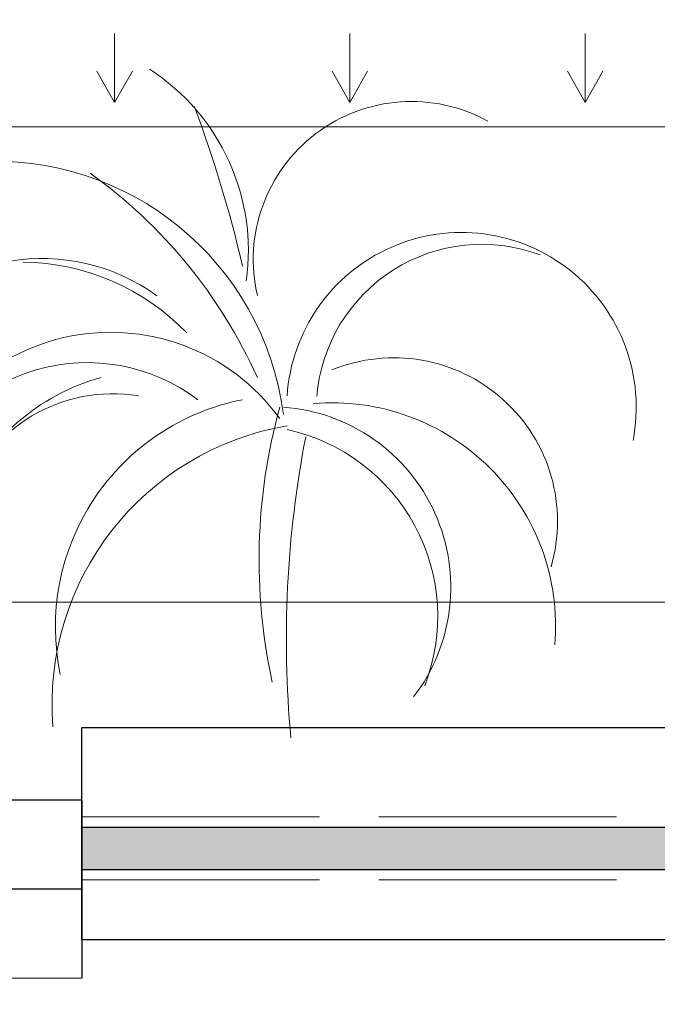
# Model space of a CAD drawing. Units: millimetres. Extents: x 595116 to 630915, y 909473 to 920225.
# Tile 31 of 134: x 629622 to 629654, y 919141 to 919190. Entities that reach past the tile are written whole.
import ezdxf

# ---------------------------------------------------------------- set-up
doc = ezdxf.new("R2010")
doc.units = ezdxf.units.MM
doc.linetypes.add('ACAD_ISO02W100', pattern=[15, 12, -3])
for name, color, linetype, lineweight in [('C-PROP', 7, 'Continuous', 25), ('C-PROP-REF', 240, 'ACAD_ISO02W100', 13), ('Dimension', 3, 'Continuous', 18), ('L-PLNT', 85, 'Continuous', 13)]:
    doc.layers.add(name, color=color, linetype=linetype, lineweight=lineweight)
doc.styles.get("Standard").update_dxf_attribs({"font": 'arial.ttf'})
doc.dimstyles.new('ISO-25', dxfattribs={"dimtxt": 9, "dimasz": 6, "dimexe": 1.25, "dimexo": 0.625, "dimtad": 1, "dimlunit": 4, "dimtxsty": 'Standard', "dimcen": 2.5, "dimadec": 0, "dimazin": 0, "dimtfac": 1, "dimtmove": 0, "dimatfit": 3, "dimfxl": 1, "dimarcsym": 0})

# ---------------------------------------------------------------- blocks, each defined once
blk = doc.blocks.new('tree')
for centre, radius, start, end in [((629595.141, 919296.95), 5.184, 352.032, 57.0714), ((629569.835, 919289.496), 31.168, 13.149, 20.5076), ((629604.232, 919296.737), 3.791, 61.1347, 193.108), ((629594.259, 919292.132), 6.965, 7.4001, 94.0059), ((629589.446, 919288.922), 12.167, 24.2477, 54.3726), ((629605.429, 919293.205), 4.185, 348.9977, 176.315), ((629605.915, 919293.144), 3.963, 69.3845, 175.231), ((629595.377, 919292.044), 4.722, 54.2484, 144.2167), ((629594.88, 919291.171), 5.506, 43.8672, 89.4805), ((629597.025, 919289.989), 5.01, 36.0581, 170.6542), ((629596.464, 919289.874), 4.4, 52.9074, 159.3471), ((629603.809, 919290.469), 3.92, 343.886, 112.2662), ((629598.153, 919288.998), 5.103, 105.3576, 208.8973), ((629597.068, 919289.758), 3.768, 80.4816, 161.0664), ((629601.247, 919287.941), 5.545, 101.0419, 191.8692), ((629602.329, 919287.957), 5.355, 355.2141, 94.8217), ((629614.329, 919289.554), 13.748, 164.5925, 192.323), ((629600.849, 919288.894), 4.324, 322.5461, 85.805), ((629602.391, 919286.088), 6.769, 99.681, 184.5451), ((629600.275, 919288.191), 4.585, 338.7925, 77.6921), ((629626.813, 919287.645), 25.579, 169.0753, 185.2889)]:
    blk.add_arc(centre, radius, start, end)
blk = doc.blocks.new('LAWN-GRASS-TUFT')
blk.add_line((0.892, 3.485), (0.892, 0))
blk.add_lwpolyline([(0, 1.577), (0.892, 0), (1.785, 1.577)])
blk = doc.blocks.new('*D216')
at = {"layer": 'Defpoints', "color": 0, "transparency": 16777216}
for p in [(629505.041, 919411.828), (629743.541, 919411.928), (629743.541, 918832.378)]:
    blk.add_point(p, dxfattribs=at)
at = {"layer": 'Dimension', "color": 0, "lineweight": -2, "transparency": 16777216}
for p, q in [((629743.541, 919411.303), (629743.541, 918831.128)), ((629505.041, 919411.203), (629505.041, 918831.128)), ((629511.041, 918832.378), (629737.541, 918832.378))]:
    blk.add_line(p, q, dxfattribs=at)
at = {"layer": 'Dimension', "color": 0, "transparency": 16777216}
for points in [[(629511.041, 918833.378), (629511.041, 918831.378), (629505.041, 918832.378)], [(629737.541, 918833.378), (629737.541, 918831.378), (629743.541, 918832.378)]]:
    blk.add_solid(points, dxfattribs=at)
at = {"layer": 'Dimension', "color": 0, "transparency": 16777216, "insert": (629624.291, 918837.656), "char_height": 9, "attachment_point": 5}
blk.add_mtext('19\'-10 1/2"', dxfattribs=at)

msp = doc.modelspace()

# ---------------------------------------------------------------- hatches: boundary and pattern name
at = {"layer": 'C-PROP'}
h = msp.add_hatch(color=256, dxfattribs=at)
h.dxf.hatch_style = 1
h.paths.add_polyline_path([(629809.541, 919149.555), (629625.041, 919149.555), (629625.041, 919147.413), (629809.541, 919147.413)])

# ---------------------------------------------------------------- linework, layer by layer
for p, q in [((629625.041, 919150.928), (629511.041, 919150.928)), ((629625.041, 919150.928), (629625.041, 919141.928)), ((629625.041, 919149.555), (629809.541, 919149.555)), ((629625.041, 919147.413), (629809.541, 919147.413))]:
    msp.add_line(p, q, dxfattribs=at)
msp.add_lwpolyline([(629809.541, 919143.864), (629625.041, 919143.864), (629625.041, 919154.587), (629809.541, 919154.587)], close=True, dxfattribs=at)
msp.add_lwpolyline([(629625.041, 919146.428), (629538.041, 919146.428)], dxfattribs=at)
at = {"layer": 'C-PROP-REF'}
for p, q in [((629625.041, 919150.076), (629809.541, 919150.076)), ((629625.041, 919146.905), (629809.541, 919146.905)), ((629625.041, 919141.928), (629538.041, 919141.928))]:
    msp.add_line(p, q, dxfattribs=at)
at = {"layer": 'L-PLNT'}
for p, q in [((629535.274, 919184.917), (629800.951, 919184.917)), ((629511.274, 919160.917), (629824.951, 919160.917))]:
    msp.add_line(p, q, dxfattribs=at)

# ---------------------------------------------------------------- block references
for p in [(629625.811, 919186.14), (629637.684, 919186.14), (629649.557, 919186.14)]:
    msp.add_blockref('LAWN-GRASS-TUFT', p, dxfattribs=at)
at = {"layer": 'L-PLNT', "xscale": 2.107689410566463, "yscale": 2.107689410566463, "zscale": 2.107689410566463}
msp.add_blockref('tree', (-697368.484, -1018413.796), dxfattribs=at)

# ---------------------------------------------------------------- dimensions: what is measured, and where the dimension line sits
at = {"layer": 'Dimension'}
dim = msp.add_linear_dim(base=(629743.541, 918832.378), p1=(629505.041, 919411.828), p2=(629743.541, 919411.928), dimstyle='ISO-25', override={"dimdec": 1, "dimlfac": 1, "dimrnd": 0, "dimzin": 1, "dimdsep": 46, "dimlunit": 4, "dimfrac": 2}, dxfattribs=at)
dim.commit()
dim.dimension.update_dxf_attribs({"geometry": '*D216', "text_midpoint": (629624.291, 918837.656)})

doc.saveas('drawing.dxf')
